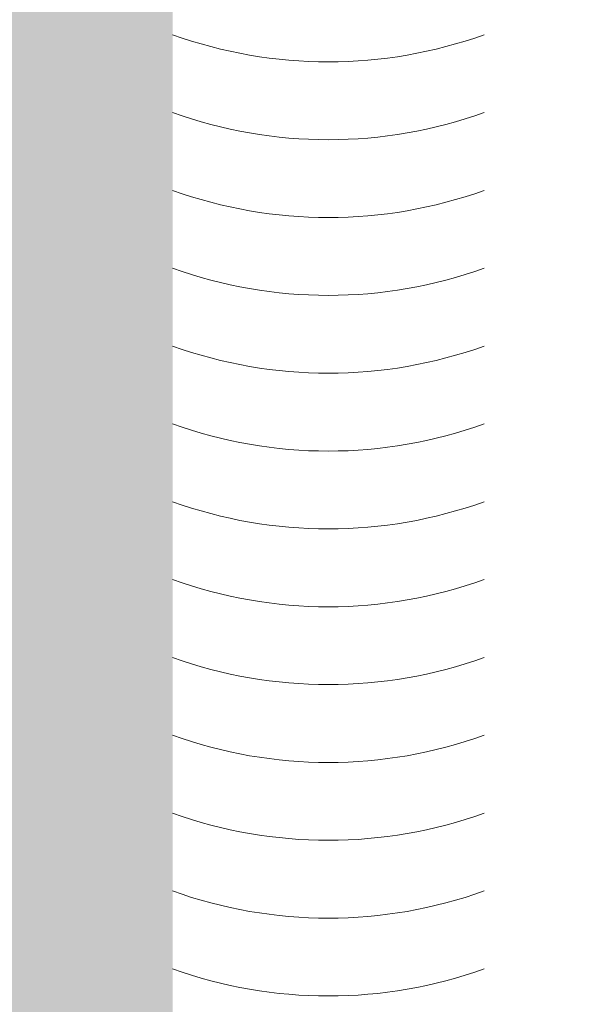
# Model space of a CAD drawing. Units: inches. Extents: x 844 to 2234, y 346 to 1084.
# Tile 86 of 93: x 2010.294 to 2012.46, y 706.497 to 710.224. Entities that reach past the tile are written whole.
import ezdxf

# ---------------------------------------------------------------- set-up
doc = ezdxf.new("R2010")
doc.units = ezdxf.units.IN
doc.header["$MEASUREMENT"] = 0
for name, color, linetype, lineweight in [('A-ANNO-DIMS', 2, 'Continuous', 18), ('furniture', 8, 'Continuous', 18), ('RA-AP-01$0$INT', 35, 'Continuous', 5)]:
    doc.layers.add(name, color=color, linetype=linetype, lineweight=lineweight)
doc.layers.add('RA-AP-01$0$FURN', color=3, linetype='Continuous')
doc.styles.get("Standard").update_dxf_attribs({"font": 'arial.ttf'})
doc.dimstyles.get("Standard").update_dxf_attribs({"dimtxt": 6, "dimasz": 3, "dimexe": 0.18, "dimexo": 0.0625, "dimgap": 0.09, "dimtad": 0, "dimtih": 1, "dimtoh": 1, "dimdec": 1, "dimzin": 0, "dimdsep": 46, "dimlunit": 3, "dimtxsty": 'Standard', "dimblk": 'ARCHTICK', "dimcen": 0.09, "dimadec": 0, "dimazin": 0, "dimtfac": 1, "dimtdec": 1, "dimtofl": 0, "dimtmove": 0, "dimatfit": 3, "dimfxl": 1, "dimtolj": 1, "dimtzin": 0, "dimarcsym": 0})

# ---------------------------------------------------------------- blocks, each defined once
blk = doc.blocks.new('A$C18D01794')
at = {"layer": 'RA-AP-01$0$INT'}
h = blk.add_hatch(color=256, dxfattribs=at)
h.paths.add_polyline_path([(4.355206456958071, -6.156712009588037), (4.355206456958071, -8.056712009588038), (5.455206456958072, -8.056712009588038), (5.455206456958072, -6.156712009588037)])
h.paths.add_polyline_path([(4.405206456958072, -8.006712009588039), (4.405206456958072, -6.206712009588038), (5.405206456958072, -6.206712009588038), (5.405206456958072, -8.006712009588039)], flags=16)
for centre in [(4.309006456954359, -7.648064458284158), (4.309006456951176, -7.671164458284799), (4.309006456954132, -7.671164458285863), (4.309006456953905, -7.694264458283548), (4.309006456953905, -7.717364458282297), (4.309006456952313, -7.740464458286957), (4.30900645695345, -7.763564458285706), (4.30900645695345, -7.786664458281272), (4.309006456951858, -7.80976445828616), (4.309006456950039, -7.832864458284682), (4.309006456952995, -7.855964458280475), (4.309006456952768, -7.879064458285135), (4.309006456951176, -7.902164458283884), (4.309006456949584, -7.925264458285589)]:
    blk.add_arc(centre, 0.136414042854523, 70.20384312815696, 109.7961568705686, dxfattribs=at)
blk = doc.blocks.new('A$C5D2F253E')
at = {"layer": 'RA-AP-01$0$FURN', "xscale": -0.7999999999883585, "yscale": 0.7999999999883585, "zscale": 0.8, "rotation": 90}
blk.add_blockref('A$C18D01794', (-5.687757199772477, 4.75791982714071), dxfattribs=at)
blk = doc.blocks.new('_ArchTick')
at = {"color": 0, "linetype": 'ByBlock', "const_width": 0.15}
blk.add_lwpolyline([(-0.5, -0.5), (0.5, 0.5)], dxfattribs=at)
blk = doc.blocks.new('*D121')
at = {"layer": 'A-ANNO-DIMS', "color": 0, "lineweight": -2, "transparency": 16777216}
for p, q in [((2030.271987351997, 734.262611118704), (2040.245275089302, 734.262611118704)), ((2040.065275089302, 734.262611118704), (2040.065275089302, 704.6043509484256)), ((2040.065275089302, 668.557359536674), (2040.065275089302, 698.2156197069523)), ((2030.271987351997, 668.557359536674), (2040.245275089302, 668.557359536674))]:
    blk.add_line(p, q, dxfattribs=at)
at = {"layer": 'Defpoints', "color": 0, "transparency": 16777216}
for p in [(2030.209487351997, 734.262611118704), (2040.065275089302, 734.262611118704), (2030.209487351997, 668.557359536674)]:
    blk.add_point(p, dxfattribs=at)
at = {"layer": 'A-ANNO-DIMS', "color": 0, "lineweight": -2, "transparency": 16777216, "xscale": 3, "yscale": 3, "zscale": 3}
for p, rotation in [((2040.065275089302, 734.262611118704), 90), ((2040.065275089302, 668.557359536674), 270)]:
    blk.add_blockref('_ArchTick', p, dxfattribs=dict(at, rotation=rotation))
at = {"layer": 'A-ANNO-DIMS', "color": 0, "transparency": 16777216, "insert": (2040.065275089302, 701.4099853276883), "char_height": 6, "attachment_point": 5}
blk.add_mtext('\\A1;LOUNGE SET 5\'-5 1/2" TYP.', dxfattribs=at)

msp = doc.modelspace()

# ---------------------------------------------------------------- block references
at = {"layer": 'furniture', "xscale": -15.94108302203742, "yscale": 15.94108302203742, "zscale": 15.94108302203742, "rotation": 270}
msp.add_blockref('A$C5D2F253E', (1990.567271852805, 701.4028671565849), dxfattribs=at)

# ---------------------------------------------------------------- dimensions: what is measured, and where the dimension line sits
at = {"layer": 'A-ANNO-DIMS'}
dim = msp.add_linear_dim(base=(2040.065275089302, 734.262611118704), p1=(2030.209487351996, 668.5573595366737), p2=(2030.209487351996, 734.2626111187037), angle=90, text='LOUNGE SET <> TYP.', dimstyle='Standard', override={"dimdec": 1, "dimlfac": 1, "dimrnd": 0, "dimzin": 1, "dimdsep": 46, "dimlunit": 4, "dimfrac": 2}, dxfattribs=at)
dim.commit()
dim.dimension.update_dxf_attribs({"geometry": '*D121', "text_midpoint": (2040.065275089302, 701.4099853276883)})

doc.saveas('drawing.dxf')
